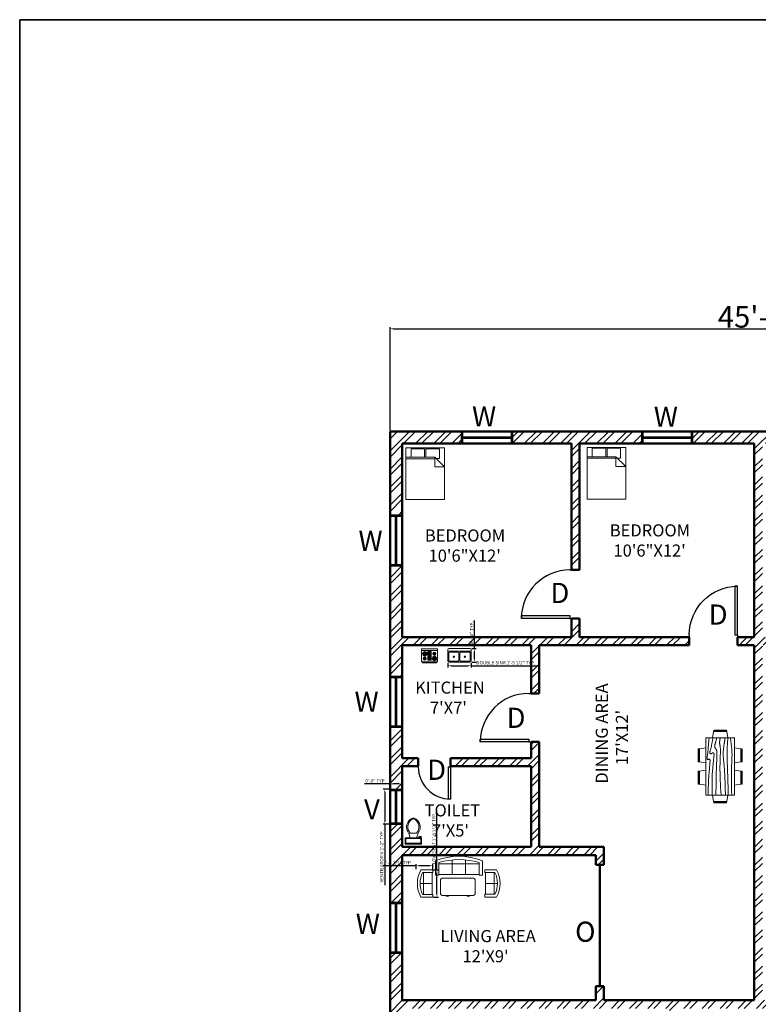
# Model space of a CAD drawing. Units: inches. Extents: x -31485 to -28799, y 18003 to 19130.
# Tile 4 of 15: x -31485 to -30936, y 18398 to 19130. Entities that reach past the tile are written whole.
import ezdxf

# ---------------------------------------------------------------- set-up
doc = ezdxf.new("R2010")
doc.units = ezdxf.units.IN
for name, color, linetype, lineweight in [('A-ANNO-DIMS', 2, 'Continuous', 18), ('A-ANNO-TEXT', 7, 'Continuous', 18), ('A-ANNO-TTLB', 7, 'Continuous', 35), ('A-AREA-IDEN', 7, 'Continuous', 18), ('A-DOOR', 3, 'Continuous', 25), ('A-FLOR-FIXT', 9, 'Continuous', 18), ('A-FURN', 8, 'Continuous', 18), ('A-GLAZ', 4, 'Continuous', 25), ('A-WALL', 7, 'Continuous', 50), ('A-WALL-PATT', 8, 'Continuous', 13)]:
    doc.layers.add(name, color=color, linetype=linetype, lineweight=lineweight)
doc.styles.get("Standard").update_dxf_attribs({"font": 'arial.ttf'})
doc.dimstyles.new('ISO-25', dxfattribs={"dimtxt": 2.5, "dimasz": 2.5, "dimexe": 1.25, "dimexo": 0.625, "dimtad": 1, "dimdec": 0, "dimlunit": 3, "dimtxsty": 'Standard', "dimcen": 2.5, "dimadec": 0, "dimazin": 0, "dimtfac": 1, "dimtdec": 0, "dimtmove": 0, "dimatfit": 3, "dimfxl": 1, "dimarcsym": 0})

# ---------------------------------------------------------------- blocks, each defined once
blk = doc.blocks.new('*U8')
for p, q in [((0, 0), (0, -100)), ((750, 0), (750, -100))]:
    blk.add_line(p, q)
blk.add_lwpolyline([(0, 0), (0, 750), (43.75, 750), (43.75, 0)], close=True)
blk.add_arc((0, 0), 750, 0, 90)
blk = doc.blocks.new('Bed - Queen')
for p, q in [((0, -80.00003), (0, 0)), ((0, 0), (59.99999, 0)), ((59.99999, 0), (59.99999, -80.00003)), ((0, -14.4), (44.8, -14.4)), ((7.99999, -1.2), (28.79998, -1.2)), ((7.99999, -14.4), (7.99999, -1.2)), ((28.79998, -1.2), (28.79998, -14.4)), ((31.19999, -1.2), (51.99999, -1.2)), ((31.19999, -14.4), (31.19999, -1.2)), ((59.99999, -29.6), (44.8, -14.4)), ((44.8, -14.4), (44.8, -29.6)), ((51.99999, -1.2), (51.99999, -16.4)), ((44.8, -16.8), (0, -16.8)), ((44.8, -29.6), (59.99999, -29.6)), ((51.99999, -16.4), (46.79936, -16.4)), ((59.99999, -80.00003), (0, -80.00003))]:
    blk.add_line(p, q)
blk = doc.blocks.new('Desk - 30 x 60 in.')
for p, q in [((-26.999995, 0), (26.999995, 0)), ((-29.999995, -27), (-29.999995, -3)), ((29.999995, -3), (29.999995, -27)), ((26.999995, -30), (-26.999995, -30)), ((-20.000005, -30), (-20.000005, -31)), ((-20.000005, -31), (-16.000005, -31)), ((-16.000005, -31), (-16.000005, -30)), ((15.999995, -31), (15.999995, -30)), ((19.999995, -31), (15.999995, -31)), ((19.999995, -30), (19.999995, -31))]:
    blk.add_line(p, q)
for centre, start, end in [((-26.499995, -3.5), 98.1301, 171.8699), ((26.499995, -3.5), 8.130102, 81.8699), ((-26.499995, -26.5), 188.1301, 261.8699), ((26.499995, -26.5), 278.1301, 351.8699)]:
    blk.add_arc(centre, 3.535534, start, end)
blk = doc.blocks.new('Sofa - Roundback 7 ft.')
for p, q in [((-36.000027, -34), (-36.000027, -11.4696)), ((-35.999844, -13.3819), (35.9998, -13.3819)), ((-12.00002, -32.4421), (-12.00003, -6.5971)), ((11.99997, -32.4421), (11.99998, -6.5971)), ((35.99998, -34), (35.99998, -11.4696)), ((-36.000027, -32.4421), (35.99998, -32.4421))]:
    blk.add_line(p, q)
for points in [[(-36.000027, -34), (-42.000027, -34), (-42.000027, -8)], [(41.99998, -8), (41.99998, -34), (35.99998, -34)]]:
    blk.add_lwpolyline(points)
for centre, radius, start, end in [((0, -114.25), 114.25, 68.43141, 111.5686), ((-0.00001, -127.1968), 121.1968, 72.72033, 107.2797)]:
    blk.add_arc(centre, radius, start, end)
blk = doc.blocks.new('Sofa - Roundback Loveseat 5 ft.')
for p, q in [((-24, -33.99998), (-24, -11.46958)), ((-23.9998, -13.38178), (23.99986, -13.38178)), ((0, -32.44198), (0, -5.99998)), ((24.00004, -33.99998), (24.00004, -11.46958)), ((-24, -32.44198), (24.00004, -32.44198))]:
    blk.add_line(p, q)
for points in [[(-24, -33.99998), (-30, -33.99998), (-30, -7.99998)], [(30.00004, -7.99998), (30.00004, -33.99998), (24.00004, -33.99998)]]:
    blk.add_lwpolyline(points)
for centre, radius, start, end in [((0, -60.24998), 60.24998, 60.13715, 119.8628), ((0, -61.38438), 55.38444, 64.32083, 115.6792)]:
    blk.add_arc(centre, radius, start, end)
blk = doc.blocks.new('Dining Set - 36 x 72 in.')
for p, q in [((-22.2343, 26.00059), (-23.4847, 17.99762)), ((-22.2304, 26), (-5.7608, 26)), ((-22, 27.5), (-22.1562, 26.50042)), ((-5.8416, 26.5), (-22.1534, 26.5)), ((-22, 27.5), (-6, 27.5)), ((-5.8437, 26.49966), (-6, 27.5)), ((-4.5152, 17.99762), (-5.7655, 25.99926)), ((5.7657, 26.00059), (4.5153, 17.99762)), ((5.7696, 26), (22.2392, 26)), ((6, 27.5), (5.8438, 26.50042)), ((22.1584, 26.5), (5.8466, 26.5)), ((6, 27.5), (22, 27.5)), ((22.1563, 26.49966), (22, 27.5)), ((23.4848, 17.99762), (22.2345, 25.99926)), ((36, 18), (-36, 18)), ((-36, 18), (-36, -18)), ((36, -18), (36, 18)), ((-45.5, 8), (-44.5004, 8.15617)), ((-45.5, 8), (-45.5, -8)), ((-44.5, -8.15843), (-44.5, 8.15338)), ((-44.0006, 8.23428), (-35.9976, 9.48474)), ((-44, 8.23041), (-44, -8.23915)), ((44.0006, 8.23428), (35.9976, 9.48474)), ((44, 8.23041), (44, -8.23915)), ((44.5, -8.15843), (44.5, 8.15338)), ((45.5, 8), (44.5005, 8.15617)), ((45.5, 8), (45.5, -8)), ((-44.4997, -8.15631), (-45.5, -8)), ((-35.9976, -9.48476), (-43.9993, -8.2345)), ((35.9976, -9.48476), (43.9993, -8.2345)), ((44.4997, -8.15631), (45.5, -8)), ((-36, -18), (36, -18)), ((-22.2343, -26.0006), (-23.4847, -17.99762)), ((-4.5152, -17.99762), (-5.7655, -25.99928)), ((5.7657, -26.0006), (4.5153, -17.99762)), ((23.4848, -17.99762), (22.2345, -25.99928)), ((-22.2304, -26), (-5.7608, -26)), ((-22, -27.5), (-22.1562, -26.50044)), ((-5.8416, -26.5), (-22.1534, -26.5)), ((-22, -27.5), (-6, -27.5)), ((-5.8437, -26.49967), (-6, -27.5)), ((5.7696, -26), (22.2392, -26)), ((6, -27.5), (5.8438, -26.50044)), ((22.1584, -26.5), (5.8466, -26.5)), ((6, -27.5), (22, -27.5)), ((22.1563, -26.49967), (22, -27.5))]:
    blk.add_line(p, q)
for points in [[(-36, 15), (-31.1772, 14.97754), (-26.8079, 14.91406), (-22.8538, 14.81543), (-19.276, 14.6875), (-16.0362, 14.53613), (-13.0957, 14.36718), (-10.4159, 14.18652), (-7.9583, 14), (-5.6904, 13.81315), (-3.6035, 13.63021), (-1.6954, 13.45508), (0.0365, 13.29166), (1.5945, 13.14388), (2.9811, 13.01562), (4.1988, 12.9108), (5.25, 12.83333), (6.1393, 12.78613), (6.8802, 12.76823), (7.4883, 12.77767), (7.9792, 12.8125), (8.3685, 12.87077), (8.6719, 12.95052), (8.9049, 13.0498), (9.0833, 13.16666), (9.2205, 13.29899), (9.3216, 13.44401), (9.3895, 13.59879), (9.4271, 13.76041), (9.4373, 13.92594), (9.4232, 14.09245), (9.3875, 14.257), (9.3333, 14.41666), (9.2638, 14.56917), (9.1836, 14.71484), (9.0975, 14.85465), (9.0104, 14.98958), (8.9272, 15.1206), (8.8529, 15.2487), (8.7922, 15.37483), (8.75, 15.5), (8.7305, 15.62467), (8.7344, 15.74739), (8.7617, 15.86621), (8.8125, 15.97916), (8.8867, 16.08431), (8.9844, 16.17968), (9.1055, 16.26334), (9.25, 16.33333), (9.4189, 16.38802), (9.6172, 16.42708), (9.8506, 16.45052), (10.125, 16.45833), (10.4463, 16.45052), (10.8203, 16.42708), (11.2529, 16.38802), (11.75, 16.33333), (12.3184, 16.26318), (12.9694, 16.17838), (13.7151, 16.07991), (14.5677, 15.96875), (15.5395, 15.84586), (16.6426, 15.71224), (17.8893, 15.56884), (19.2917, 15.41666), (20.859, 15.25667), (22.5879, 15.08984), (24.4721, 14.91715), (26.5052, 14.73958), (28.6809, 14.5581), (30.9929, 14.3737), (33.4347, 14.18733), (36, 14)], [(-36, 10), (-28.9766, 10.14274), (-23.1725, 10.20442), (-18.4241, 10.19775), (-14.5677, 10.13541), (-11.4399, 10.03011), (-8.877, 9.89453), (-6.7154, 9.74137), (-4.7917, 9.58333), (-2.9698, 9.43082), (-1.2246, 9.28515), (0.4415, 9.14534), (2.026, 9.01041), (3.5266, 8.87939), (4.9408, 8.7513), (6.266, 8.62516), (7.5, 8.5), (8.6411, 8.37549), (9.6914, 8.2539), (10.6538, 8.13818), (11.5312, 8.03125), (12.3267, 7.93603), (13.043, 7.85547), (13.6831, 7.79248), (14.25, 7.75), (14.7471, 7.7303), (15.1797, 7.73307), (15.5537, 7.75732), (15.875, 7.80208), (16.1494, 7.86637), (16.3828, 7.94922), (16.5811, 8.04964), (16.75, 8.16666), (16.8944, 8.29915), (17.0143, 8.44531), (17.1089, 8.60319), (17.1771, 8.77083), (17.218, 8.94629), (17.2305, 9.1276), (17.2137, 9.31282), (17.1667, 9.5), (17.0895, 9.6875), (16.987, 9.875), (16.8649, 10.0625), (16.7292, 10.25), (16.5856, 10.4375), (16.4401, 10.625), (16.2985, 10.8125), (16.1667, 11), (16.05, 11.18733), (15.9518, 11.3737), (15.8752, 11.5581), (15.8229, 11.73958), (15.798, 11.91715), (15.8034, 12.08984), (15.842, 12.25667), (15.9167, 12.41666), (16.0295, 12.56836), (16.1784, 12.70833), (16.3605, 12.83268), (16.5729, 12.9375), (16.8127, 13.01888), (17.0768, 13.07291), (17.3625, 13.0957), (17.6667, 13.08333), (17.9894, 13.03312), (18.3418, 12.94726), (18.7382, 12.82918), (19.1927, 12.68229), (19.7195, 12.51001), (20.3327, 12.31575), (21.0465, 12.10294), (21.875, 11.875), (22.8357, 11.63354), (23.959, 11.37304), (25.2786, 11.08618), (26.8282, 10.76562), (28.6414, 10.40405), (30.752, 9.99414), (33.1936, 9.52856), (36, 9)], [(-36, 5.5), (-30.7157, 5.3348), (-26.069, 5.20963), (-21.9946, 5.11767), (-18.4271, 5.05208), (-15.3009, 5.00602), (-12.5508, 4.97265), (-10.1112, 4.94515), (-7.9167, 4.91666), (-5.909, 4.88167), (-4.0586, 4.83984), (-2.3429, 4.79215), (-0.7396, 4.73958), (0.7739, 4.6831), (2.22, 4.6237), (3.6213, 4.56233), (5, 4.5), (6.373, 4.43782), (7.7344, 4.3776), (9.0723, 4.32129), (10.375, 4.27083), (11.6309, 4.22819), (12.8281, 4.19531), (13.9551, 4.17415), (15, 4.16666), (15.954, 4.17448), (16.819, 4.19791), (17.6001, 4.23698), (18.3021, 4.29166), (18.9299, 4.36198), (19.4883, 4.44791), (19.9823, 4.54948), (20.4167, 4.66666), (20.7969, 4.79899), (21.1302, 4.94401), (21.4245, 5.09879), (21.6875, 5.26041), (21.9271, 5.42594), (22.1511, 5.59245), (22.3672, 5.757), (22.5834, 5.91666), (22.8065, 6.06868), (23.0404, 6.21093), (23.2879, 6.34147), (23.5521, 6.45833), (23.8358, 6.55957), (24.142, 6.64323), (24.4735, 6.70735), (24.8334, 6.75), (25.2235, 6.76969), (25.642, 6.76692), (26.0858, 6.74267), (26.5521, 6.69791), (27.0379, 6.63362), (27.5404, 6.55078), (28.0565, 6.45036), (28.5834, 6.33333), (29.1242, 6.19987), (29.7071, 6.04687), (30.3661, 5.87044), (31.1354, 5.66666), (32.0493, 5.43164), (33.142, 5.16146), (34.4475, 4.85221), (36, 4.5)], [(-36, -1), (-30.7915, -0.6591), (-26.0195, -0.38216), (-21.6519, -0.16284), (-17.6563, 0.00521), (-14.0005, 0.12833), (-10.6523, 0.21289), (-7.5796, 0.26522), (-4.75, 0.29166), (-2.134, 0.29793), (0.2878, 0.28711), (2.5317, 0.26163), (4.6146, 0.22396), (6.5529, 0.17651), (8.3633, 0.12174), (10.0623, 0.06209), (11.6667, 0), (13.1899, -0.06201), (14.6341, -0.1211), (15.9982, -0.17432), (17.2813, -0.21875), (18.4823, -0.25147), (19.6003, -0.26953), (20.6343, -0.27002), (21.5834, -0.25), (22.4481, -0.20768), (23.2357, -0.14584), (23.9549, -0.06836), (24.6146, 0.02083), (25.2235, 0.11784), (25.7904, 0.21875), (26.3241, 0.31966), (26.8334, 0.41666), (27.3265, 0.50618), (27.8099, 0.58593), (28.2894, 0.65397), (28.7709, 0.70833), (29.2601, 0.74707), (29.763, 0.76823), (30.2855, 0.76985), (30.8334, 0.75), (31.4088, 0.70784), (31.9994, 0.64713), (32.589, 0.57275), (33.1615, 0.48958), (33.7008, 0.4025), (34.1908, 0.3164), (34.6153, 0.23616), (34.9584, 0.16666), (35.2099, 0.11165), (35.3848, 0.07031), (35.504, 0.04069), (35.5886, 0.02083), (35.6594, 0.00879), (35.7377, 0.0026), (35.8442, 0.00032), (36, 0)], [(-36, -6.5), (-27.1843, -6.31267), (-20.084, -6.1263), (-14.469, -5.9419), (-10.1094, -5.76042), (-6.7752, -5.58285), (-4.2363, -5.41016), (-2.2629, -5.24333), (-0.625, -5.08334), (0.8708, -4.93099), (2.2715, -4.78646), (3.5872, -4.64974), (4.8281, -4.52084), (6.0046, -4.39974), (7.127, -4.28646), (8.2053, -4.18099), (9.25, -4.08334), (10.2705, -3.99382), (11.2734, -3.91407), (12.2647, -3.84603), (13.25, -3.79167), (14.2354, -3.75293), (15.2266, -3.73177), (16.2295, -3.73015), (17.25, -3.75), (18.2912, -3.79248), (19.3451, -3.85547), (20.4009, -3.93604), (21.4479, -4.03125), (22.4754, -4.13819), (23.4727, -4.25391), (24.4289, -4.37549), (25.3334, -4.5), (26.1785, -4.62492), (26.9694, -4.74935), (27.7145, -4.87281), (28.4219, -4.99479), (29.1, -5.11483), (29.7572, -5.23242), (30.4016, -5.34709), (31.0417, -5.45834), (31.6837, -5.56437), (32.3262, -5.65821), (32.9658, -5.73153), (33.599, -5.77604), (34.2224, -5.78345), (34.8327, -5.74545), (35.4264, -5.65373), (36, -5.5)], [(-36, -10), (-26.4022, -9.81299), (-18.4675, -9.62891), (-11.9839, -9.45069), (-6.7396, -9.28125), (-2.5226, -9.12354), (0.8789, -8.98047), (3.6769, -8.85498), (6.0833, -8.75), (8.2767, -8.66765), (10.3021, -8.60677), (12.1712, -8.56543), (13.8958, -8.54167), (15.4876, -8.53353), (16.9583, -8.53907), (18.3197, -8.55632), (19.5834, -8.58334), (20.7616, -8.61841), (21.8685, -8.66081), (22.9188, -8.71004), (23.9271, -8.76563), (24.9081, -8.82707), (25.8763, -8.89388), (26.8465, -8.96558), (27.8334, -9.04167), (28.8474, -9.12118), (29.8828, -9.20117), (30.93, -9.27824), (31.9792, -9.34896), (33.0205, -9.40991), (34.0443, -9.45768), (35.0407, -9.48885), (36, -9.5)], [(-36, -14.5), (-30.0881, -14.33513), (-25.0332, -14.21224), (-20.7312, -14.12647), (-17.0781, -14.07292), (-13.97, -14.04671), (-11.3027, -14.04297), (-8.9724, -14.05681), (-6.875, -14.08334), (-4.9224, -14.11833), (-3.0905, -14.16016), (-1.3709, -14.20785), (0.2448, -14.26042), (1.7647, -14.3169), (3.1973, -14.3763), (4.5507, -14.43767), (5.8333, -14.5), (7.0554, -14.5621), (8.235, -14.62175), (9.3922, -14.67652), (10.5469, -14.72396), (11.7192, -14.76164), (12.929, -14.78711), (14.1965, -14.79794), (15.5417, -14.79167), (16.9933, -14.76424), (18.6152, -14.70508), (20.4804, -14.60197), (22.6615, -14.44271), (25.2312, -14.21509), (28.2624, -13.9069), (31.8277, -13.50594), (36, -13)]]:
    blk.add_lwpolyline(points)
blk = doc.blocks.new('Range-Oven - 30 in top')
for p, q in [((0, -3), (30, -3)), ((12, -6), (18, -6)), ((13, -20), (13, -6)), ((14, -6), (14, -20)), ((15, -20), (15, -6)), ((16, -6), (16, -20)), ((17, -20), (17, -6)), ((6, -24), (6, -25)), ((8, -25), (8, -24)), ((18, -20), (12, -20)), ((22, -25), (22, -24)), ((24, -24), (24, -25))]:
    blk.add_line(p, q)
for points in [[(0, -24), (0, 0), (30, 0), (30, -24)], [(12, -21), (12, -5), (18, -5), (18, -21)], [(2, -26), (2, -25), (28, -25), (28, -26)]]:
    blk.add_lwpolyline(points, close=True)
for centre, radius in [((6, -9), 4), ((6, -9), 3), ((6, -18), 3), ((6, -9), 2), ((6, -18), 2), ((6, -9), 1), ((6, -18), 1), ((24, -18), 4), ((24, -9), 3), ((24, -18), 3), ((24, -9), 2), ((24, -18), 2), ((24, -9), 1), ((24, -18), 1)]:
    blk.add_circle(centre, radius)
blk = doc.blocks.new('Sink-double - 36 in top')
for p, q in [((-18, -4), (18, -4)), ((-0.75, -18.5), (-0.75, -6.5)), ((0.75, -6.5), (0.75, -18.5))]:
    blk.add_line(p, q)
for points in [[(-16.5, 0), (16.5, 0)], [(-18, -19.5), (-18, -1.5)], [(-16.5, -18.5), (-16.5, -6.5)], [(-15.5, -5.5), (-1.75, -5.5)], [(1.75, -5.5), (15.5, -5.5)], [(16.5, -6.5), (16.5, -18.5)], [(18, -1.5), (18, -19.5)], [(16.5, -21), (-16.5, -21)], [(-1.75, -19.5), (-15.5, -19.5)], [(15.5, -19.5), (1.75, -19.5)]]:
    blk.add_lwpolyline(points)
for centre, radius in [((-8.5, -12.5), 1), ((-8.5, -12.5), 0.5), ((8.5, -12.5), 1), ((8.5, -12.5), 0.5)]:
    blk.add_circle(centre, radius)
for centre, radius, start, end in [((-16.5, -1.5), 1.5, 90, 180), ((16.5, -1.5), 1.5, 0, 90), ((-15.5, -6.5), 1, 90, 180), ((-1.75, -6.5), 1, 0, 90), ((1.75, -6.5), 1, 90, 180), ((15.5, -6.5), 1, 0, 90), ((-16.5, -19.5), 1.5, 180, 270), ((-15.5, -18.5), 1, 180, 270), ((-1.75, -18.5), 1, 270, 0), ((1.75, -18.5), 1, 180, 270), ((15.5, -18.5), 1, 270, 0), ((16.5, -19.5), 1.5, 270, 0)]:
    blk.add_arc(centre, radius, start, end)
blk = doc.blocks.new('Toilet - top')
for p, q in [((-10, -8.5), (-8, -8.5)), ((-10, -9.5), (-10, -8.5)), ((-7, -9.5), (-10, -9.5)), ((-8, -8.5), (-8, -8)), ((-7, -8), (-7, -9.5)), ((-4, -8), (-6, -14)), ((4, -8), (6, -14)), ((9.5, -6), (9.5, -2)), ((4, -14), (-4, -14))]:
    blk.add_line(p, q)
blk.add_lwpolyline([(10.5, -8), (10.5, 0), (-10.5, 0), (-10.5, -8)], close=True)
for points in [[(-9.5, -2), (-9.5, -6)], [(8.5, -1), (-8.5, -1)], [(-8.5, -7), (8.5, -7)]]:
    blk.add_lwpolyline(points)
for centre, radius, start, end in [((-8.6, -1.9), 0.884, 81.8699, 188.1301), ((-8.6, -6.1), 0.884, 171.8699, 278.1301), ((8.6, -1.9), 0.884, 351.8699, 98.1301), ((8.6, -6.1), 0.884, 261.8699, 8.1301), ((3.5, -21.6), 12.2, 141.4691, 247.9714), ((4.2, -21.8), 11.3, 136.3677, 238.9468), ((-3.5, -21.6), 12.2, 292.0284, 38.5307), ((-4.2, -21.8), 11.3, 301.053, 43.6321), ((0, -27.9), 4, 245.7318, 294.2682), ((0, -29), 4, 254.8605, 285.1395)]:
    blk.add_arc(centre, radius, start, end)
blk = doc.blocks.new('*D200')
at = {"layer": 'A-ANNO-DIMS', "color": 0, "lineweight": -2, "transparency": 16777216}
for p, q in [((-31209.53, 18824.43), (-31209.53, 18901.41)), ((-31207.03, 18900.16), (-30664.03, 18900.16)), ((-30661.53, 18824.43), (-30661.53, 18901.41))]:
    blk.add_line(p, q, dxfattribs=at)
at = {"layer": 'A-ANNO-DIMS', "color": 0, "transparency": 16777216}
for points in [[(-31207.03, 18900.58), (-31207.03, 18899.75), (-31209.53, 18900.16)], [(-30664.03, 18900.58), (-30664.03, 18899.75), (-30661.53, 18900.16)]]:
    blk.add_solid(points, dxfattribs=at)
at = {"layer": 'Defpoints', "color": 0, "transparency": 16777216}
for p in [(-30661.53, 18900.16), (-31209.53, 18823.8), (-30661.53, 18823.8)]:
    blk.add_point(p, dxfattribs=at)
at = {"layer": 'A-ANNO-DIMS', "color": 0, "transparency": 16777216, "insert": (-30935.53, 18908.96), "char_height": 2.5, "attachment_point": 5}
blk.add_mtext('{\\H6.4x;45\'-8"}', dxfattribs=at)
blk = doc.blocks.new('WIN-900-W9')
for p, q in [((-29982.21, 18824.12), (-29982.21, 18815.12)), ((-29981.21, 18824.12), (-29981.21, 18815.12)), ((-29945.21, 18824.12), (-29945.21, 18815.12)), ((-29944.21, 18824.12), (-29944.21, 18815.12)), ((-29981.21, 18820.12), (-29945.21, 18820.12)), ((-29981.21, 18819.62), (-29945.21, 18819.62)), ((-29981.21, 18819.12), (-29945.21, 18819.12))]:
    blk.add_line(p, q)
blk = doc.blocks.new('VENT-600-W9')
for p, q in [((-29896.21, 18594.12), (-29905.21, 18594.12)), ((-29896.21, 18593.12), (-29905.21, 18593.12)), ((-29901.21, 18593.12), (-29901.21, 18569.12)), ((-29900.71, 18593.12), (-29900.71, 18569.12)), ((-29900.21, 18593.12), (-29900.21, 18569.12)), ((-29896.21, 18569.12), (-29905.21, 18569.12)), ((-29896.21, 18568.12), (-29905.21, 18568.12))]:
    blk.add_line(p, q)
blk = doc.blocks.new('*D216')
at = {"layer": 'A-ANNO-DIMS', "color": 0, "lineweight": -2, "transparency": 16777216}
for p, q in [((-31210.15, 18557.8), (-31214.68, 18557.8)), ((-31213.43, 18555.3), (-31213.43, 18534.3)), ((-31210.15, 18531.8), (-31214.68, 18531.8)), ((-31213.43, 18531.8), (-31213.43, 18486.49))]:
    blk.add_line(p, q, dxfattribs=at)
at = {"layer": 'A-ANNO-DIMS', "color": 0, "transparency": 16777216}
for points in [[(-31213.84, 18555.3), (-31213.01, 18555.3), (-31213.43, 18557.8)], [(-31213.84, 18534.3), (-31213.01, 18534.3), (-31213.43, 18531.8)]]:
    blk.add_solid(points, dxfattribs=at)
at = {"layer": 'Defpoints', "color": 0, "transparency": 16777216}
for p in [(-31209.53, 18557.8), (-31213.43, 18531.8), (-31209.53, 18531.8)]:
    blk.add_point(p, dxfattribs=at)
at = {"layer": 'A-ANNO-DIMS', "color": 0, "transparency": 16777216, "insert": (-31215.35, 18507.89), "char_height": 2.5, "attachment_point": 5, "rotation": 90}
blk.add_mtext('VENTILATOR V 2\'-2" TYP.', dxfattribs=at)
blk = doc.blocks.new('*D217')
at = {"layer": 'A-ANNO-DIMS', "color": 0, "lineweight": -2, "transparency": 16777216}
for p, q in [((-31209.53, 18561.7), (-31228.52, 18561.7)), ((-31209.53, 18558.43), (-31209.53, 18562.95)), ((-31203.03, 18561.7), (-31207.03, 18561.7)), ((-31200.53, 18558.43), (-31200.53, 18562.95))]:
    blk.add_line(p, q, dxfattribs=at)
at = {"layer": 'A-ANNO-DIMS', "color": 0, "transparency": 16777216}
for points in [[(-31207.03, 18562.12), (-31207.03, 18561.29), (-31209.53, 18561.7)], [(-31203.03, 18562.12), (-31203.03, 18561.29), (-31200.53, 18561.7)]]:
    blk.add_solid(points, dxfattribs=at)
at = {"layer": 'Defpoints', "color": 0, "transparency": 16777216}
for p in [(-31209.53, 18561.7), (-31209.53, 18557.8), (-31200.53, 18557.8)]:
    blk.add_point(p, dxfattribs=at)
at = {"layer": 'A-ANNO-DIMS', "color": 0, "transparency": 16777216, "insert": (-31220.27, 18563.6), "char_height": 2.5, "attachment_point": 5}
blk.add_mtext('0\'-9" TYP.', dxfattribs=at)
blk = doc.blocks.new('*D226')
at = {"layer": 'A-ANNO-DIMS', "color": 0, "lineweight": -2, "transparency": 16777216}
for p, q in [((-31174.67, 18497.78), (-31174.67, 18541.89)), ((-31177.09, 18497.78), (-31173.42, 18497.78)), ((-31174.67, 18479.99), (-31174.67, 18495.28)), ((-31177.09, 18477.49), (-31173.42, 18477.49))]:
    blk.add_line(p, q, dxfattribs=at)
at = {"layer": 'A-ANNO-DIMS', "color": 0, "transparency": 16777216}
for points in [[(-31175.08, 18495.28), (-31174.25, 18495.28), (-31174.67, 18497.78)], [(-31175.08, 18479.99), (-31174.25, 18479.99), (-31174.67, 18477.49)]]:
    blk.add_solid(points, dxfattribs=at)
at = {"layer": 'Defpoints', "color": 0, "transparency": 16777216}
for p in [(-31177.71, 18497.78), (-31174.67, 18497.78), (-31177.71, 18477.49)]:
    blk.add_point(p, dxfattribs=at)
at = {"layer": 'A-ANNO-DIMS', "color": 0, "transparency": 16777216, "insert": (-31176.59, 18521.08), "char_height": 2.5, "attachment_point": 5, "rotation": 90}
blk.add_mtext('LOVESEAT 1\'-8 1/2" TYP.', dxfattribs=at)
blk = doc.blocks.new('*D227')
at = {"layer": 'A-ANNO-DIMS', "color": 0, "lineweight": -2, "transparency": 16777216}
for p, q in [((-31190.11, 18498.4), (-31190.11, 18502.07)), ((-31177.71, 18498.4), (-31177.71, 18502.07)), ((-31190.11, 18500.82), (-31214.69, 18500.82)), ((-31180.21, 18500.82), (-31187.61, 18500.82))]:
    blk.add_line(p, q, dxfattribs=at)
at = {"layer": 'A-ANNO-DIMS', "color": 0, "transparency": 16777216}
for points in [[(-31187.61, 18501.24), (-31187.61, 18500.4), (-31190.11, 18500.82)], [(-31180.21, 18501.24), (-31180.21, 18500.4), (-31177.71, 18500.82)]]:
    blk.add_solid(points, dxfattribs=at)
at = {"layer": 'Defpoints', "color": 0, "transparency": 16777216}
for p in [(-31190.11, 18500.82), (-31190.11, 18497.78), (-31177.71, 18497.78)]:
    blk.add_point(p, dxfattribs=at)
at = {"layer": 'A-ANNO-DIMS', "color": 0, "transparency": 16777216, "insert": (-31203.65, 18502.74), "char_height": 2.5, "attachment_point": 5}
blk.add_mtext('1\'-0 1/2" TYP.', dxfattribs=at)
blk = doc.blocks.new('*D254')
at = {"layer": 'A-ANNO-DIMS', "color": 0, "lineweight": -2, "transparency": 16777216}
for p, q in [((-31166.61, 18651.53), (-31166.61, 18648.3)), ((-31164.11, 18649.55), (-31151.75, 18649.55)), ((-31149.25, 18651.53), (-31149.25, 18648.3)), ((-31149.25, 18649.55), (-31100.1, 18649.55))]:
    blk.add_line(p, q, dxfattribs=at)
at = {"layer": 'A-ANNO-DIMS', "color": 0, "transparency": 16777216}
for points in [[(-31164.11, 18649.96), (-31164.11, 18649.13), (-31166.61, 18649.55)], [(-31151.75, 18649.96), (-31151.75, 18649.13), (-31149.25, 18649.55)]]:
    blk.add_solid(points, dxfattribs=at)
at = {"layer": 'Defpoints', "color": 0, "transparency": 16777216}
for p in [(-31166.61, 18652.15), (-31149.25, 18652.15), (-31149.25, 18649.55)]:
    blk.add_point(p, dxfattribs=at)
at = {"layer": 'A-ANNO-DIMS', "color": 0, "transparency": 16777216, "insert": (-31123.42, 18651.46), "char_height": 2.5, "attachment_point": 5}
blk.add_mtext('DOUBLE SINK 1\'-5 1/2" TYP.', dxfattribs=at)
blk = doc.blocks.new('*D255')
at = {"layer": 'A-ANNO-DIMS', "color": 0, "lineweight": -2, "transparency": 16777216}
for p, q in [((-31146.64, 18662.28), (-31146.64, 18683.21)), ((-31148.62, 18662.28), (-31145.39, 18662.28)), ((-31146.64, 18654.65), (-31146.64, 18659.78)), ((-31148.62, 18652.15), (-31145.39, 18652.15))]:
    blk.add_line(p, q, dxfattribs=at)
at = {"layer": 'A-ANNO-DIMS', "color": 0, "transparency": 16777216}
for points in [[(-31147.06, 18659.78), (-31146.23, 18659.78), (-31146.64, 18662.28)], [(-31147.06, 18654.65), (-31146.23, 18654.65), (-31146.64, 18652.15)]]:
    blk.add_solid(points, dxfattribs=at)
at = {"layer": 'Defpoints', "color": 0, "transparency": 16777216}
for p in [(-31149.25, 18662.28), (-31146.64, 18662.28), (-31149.25, 18652.15)]:
    blk.add_point(p, dxfattribs=at)
at = {"layer": 'A-ANNO-DIMS', "color": 0, "transparency": 16777216, "insert": (-31148.54, 18674), "char_height": 2.5, "attachment_point": 5, "rotation": 90}
blk.add_mtext('0\'-10" TYP.', dxfattribs=at)

msp = doc.modelspace()

# ---------------------------------------------------------------- hatches: boundary and pattern name
at = {"layer": 'A-WALL-PATT'}
h = msp.add_hatch(dxfattribs=at)
h.set_pattern_fill('ANSI32', color=256)
h.set_pattern_definition([(45, (-1687.357, -0.313), (-6.735192, 6.735192), []), (45, (-1682.867, -0.313), (-6.735192, 6.735192), [])])
h.paths.add_polyline_path([(-31156.53, 18823.8), (-31209.53, 18823.8), (-31209.53, 18761.8), (-31200.53, 18761.8), (-31200.53, 18814.8), (-31156.53, 18814.8)], flags=17)
h.paths.add_polyline_path([(-31022.53, 18823.8), (-31118.53, 18823.8), (-31118.53, 18814.8), (-31074.53, 18814.8), (-31074.53, 18720.79), (-31070.96, 18720.79), (-31068.53, 18720.76), (-31068.53, 18814.8), (-31022.53, 18814.8)], flags=17)
h.paths.add_polyline_path([(-30754.53, 18823.8), (-30850.53, 18823.8), (-30850.53, 18814.8), (-30806.53, 18814.8), (-30806.53, 18723.1), (-30800.53, 18723.1), (-30800.53, 18814.8), (-30754.53, 18814.8)], flags=17)
h.paths.add_polyline_path([(-30661.53, 18823.8), (-30716.53, 18823.8), (-30716.53, 18814.8), (-30670.53, 18814.8), (-30670.53, 18761.8), (-30661.53, 18761.8)], flags=17)
h.paths.add_polyline_path([(-30986.92, 18670.8), (-31068.53, 18670.8), (-31068.53, 18684.76), (-31074.53, 18684.76), (-31074.53, 18670.8), (-31200.53, 18670.8), (-31200.53, 18723.8), (-31209.53, 18723.8), (-31209.53, 18641.8), (-31200.53, 18641.8), (-31200.53, 18664.8), (-31104.53, 18664.8), (-31104.53, 18628.93), (-31098.53, 18628.93), (-31098.53, 18664.8), (-30986.92, 18664.8)], flags=17)
h.paths.add_polyline_path([(-30661.53, 18723.8), (-30670.53, 18723.8), (-30670.53, 18670.8), (-30800.53, 18670.8), (-30800.53, 18687.1), (-30806.53, 18687.1), (-30806.53, 18670.8), (-30885.6, 18670.8), (-30885.6, 18667.8), (-30885.6, 18664.8), (-30760.53, 18664.8), (-30760.53, 18625.8), (-30754.53, 18625.8), (-30754.53, 18664.8), (-30670.53, 18664.8), (-30670.53, 18641.8), (-30661.53, 18641.8)], flags=17)
h.paths.add_polyline_path([(-31200.53, 18574.8), (-31188.56, 18574.8), (-31188.56, 18580.8), (-31200.53, 18580.8), (-31200.53, 18603.8), (-31209.53, 18603.8), (-31209.53, 18557.8), (-31200.53, 18557.8)], flags=17)
h.paths.add_polyline_path([(-31098.53, 18592.93), (-31104.53, 18592.93), (-31104.53, 18580.8), (-31164.56, 18580.8), (-31164.56, 18574.8), (-31104.53, 18574.8), (-31104.53, 18514.8), (-31200.53, 18514.8), (-31200.53, 18531.8), (-31209.53, 18531.8), (-31209.53, 18473.8), (-31200.53, 18473.8), (-31200.53, 18508.8), (-31056.53, 18508.8), (-31056.53, 18501.62), (-31050.53, 18501.62), (-31050.53, 18514.8), (-31098.53, 18514.8)], flags=17)
h.paths.add_polyline_path([(-30661.53, 18531.8), (-30670.53, 18531.8), (-30670.53, 18514.8), (-30754.53, 18514.8), (-30754.53, 18574.8), (-30700.75, 18574.8), (-30700.75, 18577.44), (-30700.75, 18580.8), (-30754.53, 18580.8), (-30754.53, 18589.8), (-30760.53, 18589.8), (-30760.53, 18514.8), (-30820.53, 18514.8), (-30820.53, 18499.26), (-30814.53, 18499.26), (-30814.53, 18508.8), (-30670.53, 18508.8), (-30670.53, 18473.8), (-30661.53, 18473.8)], flags=17)
h.paths.add_polyline_path([(-30661.53, 18435.8), (-30670.53, 18435.8), (-30670.53, 18400.8), (-30814.53, 18400.8), (-30814.53, 18413.15), (-30820.53, 18413.15), (-30820.53, 18400.8), (-30932.53, 18400.8), (-30932.53, 18664.8), (-30921.6, 18664.8), (-30921.6, 18670.8), (-30932.53, 18670.8), (-30932.53, 18814.8), (-30888.53, 18814.8), (-30888.53, 18823.8), (-30984.53, 18823.8), (-30984.53, 18814.8), (-30938.53, 18814.8), (-30938.53, 18670.8), (-30950.92, 18670.8), (-30950.92, 18664.8), (-30938.53, 18664.8), (-30938.53, 18400.8), (-31050.53, 18400.8), (-31050.53, 18411.18), (-31056.53, 18411.18), (-31056.53, 18400.8), (-31200.53, 18400.8), (-31200.53, 18435.8), (-31209.53, 18435.8), (-31209.53, 18179.8), (-31200.53, 18179.8), (-31200.53, 18394.8), (-31001.53, 18394.8), (-31001.53, 18179.8), (-30954.53, 18179.8), (-30954.53, 18188.8), (-30995.53, 18188.8), (-30995.53, 18394.8), (-30875.53, 18394.8), (-30875.53, 18188.8), (-30916.53, 18188.8), (-30916.53, 18179.8), (-30869.53, 18179.8), (-30869.53, 18394.8), (-30670.53, 18394.8), (-30670.53, 18179.8), (-30661.53, 18179.8)])

# ---------------------------------------------------------------- linework, layer by layer
at = {"layer": 'A-ANNO-TTLB'}
msp.add_lwpolyline([(-31485.1, 19129.94), (-28798.64, 19129.94), (-28798.64, 18002.86), (-31485.1, 18002.86)], close=True, dxfattribs=at)
at = {"layer": 'A-WALL'}
for p, q in [((-31209.53, 18823.8), (-30661.53, 18823.8)), ((-31209.53, 18179.8), (-31209.53, 18823.8)), ((-31200.53, 18814.8), (-31074.53, 18814.8)), ((-31200.53, 18670.8), (-31200.53, 18814.8)), ((-31074.53, 18720.76), (-31074.53, 18814.8)), ((-31068.53, 18814.8), (-30938.53, 18814.8)), ((-31068.53, 18720.76), (-31068.53, 18814.8)), ((-30938.53, 18814.8), (-30938.53, 18670.8)), ((-31074.53, 18720.76), (-31068.53, 18720.76)), ((-31074.53, 18670.8), (-31074.53, 18684.76)), ((-31074.53, 18684.76), (-31068.53, 18684.76)), ((-31068.53, 18670.8), (-31068.53, 18684.76)), ((-31200.53, 18670.8), (-31074.53, 18670.8)), ((-31068.53, 18670.8), (-30986.92, 18670.8)), ((-30986.92, 18670.8), (-30986.92, 18664.8)), ((-30950.92, 18670.8), (-30938.53, 18670.8)), ((-30950.92, 18670.8), (-30950.92, 18664.8)), ((-31200.53, 18664.8), (-31104.53, 18664.8)), ((-31200.53, 18580.8), (-31200.53, 18664.8)), ((-31104.53, 18628.93), (-31104.53, 18664.8)), ((-31098.53, 18664.8), (-30986.92, 18664.8)), ((-31098.53, 18628.93), (-31098.53, 18664.8)), ((-30950.92, 18664.8), (-30938.53, 18664.8)), ((-30938.53, 18664.8), (-30938.53, 18400.8)), ((-31104.53, 18628.93), (-31098.53, 18628.93)), ((-31104.53, 18580.8), (-31104.53, 18592.93)), ((-31104.53, 18592.93), (-31098.53, 18592.93)), ((-31098.53, 18514.8), (-31098.53, 18592.93)), ((-31200.53, 18580.8), (-31188.56, 18580.8)), ((-31200.53, 18574.8), (-31188.56, 18574.8)), ((-31200.53, 18514.8), (-31200.53, 18574.8)), ((-31188.56, 18580.8), (-31188.56, 18574.8)), ((-31164.56, 18580.8), (-31104.53, 18580.8)), ((-31164.56, 18580.8), (-31164.56, 18574.8)), ((-31164.56, 18574.8), (-31104.53, 18574.8)), ((-31104.53, 18514.8), (-31104.53, 18574.8)), ((-31200.53, 18514.8), (-31104.53, 18514.8)), ((-31200.53, 18508.8), (-31056.53, 18508.8)), ((-31200.53, 18400.8), (-31200.53, 18508.8)), ((-31098.53, 18514.8), (-31050.53, 18514.8)), ((-31056.53, 18501.62), (-31056.53, 18508.8)), ((-31050.53, 18501.62), (-31050.53, 18514.8)), ((-31056.53, 18501.62), (-31050.53, 18501.62)), ((-31053.53, 18501.62), (-31053.53, 18411.18)), ((-31056.53, 18400.8), (-31056.53, 18411.18)), ((-31056.53, 18411.18), (-31050.53, 18411.18)), ((-31050.53, 18400.8), (-31050.53, 18411.18)), ((-31200.53, 18400.8), (-31056.53, 18400.8)), ((-31050.53, 18400.8), (-30938.53, 18400.8))]:
    msp.add_line(p, q, dxfattribs=at)

# ---------------------------------------------------------------- block references
at = {"layer": 'A-DOOR'}
for p, xscale, yscale, zscale, rotation in [((-31075.76, 18684.74), 0.0480636078261425, 0.0480636078261425, 0.0480636078261425, 90.00000000000003), ((-31106.36, 18592.92), 0.0480122828236164, 0.0480122828236164, 0.0480122828236164, 90.00000000000003), ((-31164.56, 18574.45), 0.0319880955261889, 0.0319880955261889, 0.0319880955261889, 180)]:
    msp.add_blockref('*U8', p, dxfattribs=dict(at, xscale=xscale, yscale=yscale, zscale=zscale, rotation=rotation))
at = {"layer": 'A-DOOR', "xscale": -0.0480000000000013, "yscale": 0.0480000000000013, "zscale": 0.0480000000000013}
msp.add_blockref('*U8', (-30950.92, 18672.6), dxfattribs=at)
at = {"layer": 'A-FLOR-FIXT'}
for name, p, xscale, yscale, zscale in [('Sink-double - 36 in top', (-31157.93, 18662.28), 0.4823765274114516, 0.4823765274114516, 0.4823765274114516), ('Range-Oven - 30 in top', (-31186.15, 18662.06), 0.4, 0.4, 0.4)]:
    msp.add_blockref(name, p, dxfattribs=dict(at, xscale=xscale, yscale=yscale, zscale=zscale))
at = {"layer": 'A-FLOR-FIXT', "xscale": 0.5850068734066302, "yscale": 0.5850068734066302, "zscale": 0.5850068734066302, "rotation": 180}
msp.add_blockref('Toilet - top', (-31192.16, 18516.94), dxfattribs=at)
at = {"layer": 'A-FURN'}
for name, p, xscale, yscale, zscale in [('Bed - Queen', (-31197.75, 18811.54), 0.479364226334794, 0.479364226334794, 0.479364226334794), ('Bed - Queen', (-31062.9, 18811.85), 0.479364226334794, 0.479364226334794, 0.479364226334794), ('Sofa - Roundback 7 ft.', (-31158.28, 18507.9), 0.4147575827902149, 0.4147575827902149, 0.4147575827902149), ('Desk - 30 x 60 in.', (-31159.11, 18491.59), 0.4297812202416646, 0.4297812202416646, 0.4297812202416646)]:
    msp.add_blockref(name, p, dxfattribs=dict(at, xscale=xscale, yscale=yscale, zscale=zscale))
for name, p, xscale, yscale, zscale, rotation in [('Dining Set - 36 x 72 in.', (-30963.88, 18574.61), 0.5930176886900861, 0.5930176886900861, 0.5930176886900861, 90), ('Sofa - Roundback Loveseat 5 ft.', (-31189.21, 18487.63), 0.3381495698466857, 0.3381495698466857, 0.3381495698466857, 89.99999999999999), ('Sofa - Roundback Loveseat 5 ft.', (-31127.6, 18487.71), 0.3381495698466857, 0.3381495698466857, 0.3381495698466857, 270)]:
    msp.add_blockref(name, p, dxfattribs=dict(at, xscale=xscale, yscale=yscale, zscale=zscale, rotation=rotation))
at = {"layer": 'A-GLAZ'}
for p in [(-1174.32, -0.31), (-1040.32, -0.31)]:
    msp.add_blockref('WIN-900-W9', p, dxfattribs=at)
for name, p, rotation in [('WIN-900-W9', (-12385.41, 48706.01), 89.99999999997677), ('WIN-900-W9', (-12385.41, 48586.01), 89.9999999999743), ('VENT-600-W9', (-61105.73, 37125.92), 180), ('WIN-900-W9', (-12385.41, 48418.01), 89.9999999999743)]:
    msp.add_blockref(name, p, dxfattribs=dict(at, rotation=rotation))

# ---------------------------------------------------------------- texts
at = {"layer": 'A-ANNO-TEXT', "char_height": 15, "attachment_point": 1}
for s, insert in [('{W}', (-31148.54, 18842.45)), ('{W}', (-31013.31, 18842.27)), ('{W}', (-31233.02, 18749.96)), ('{D}', (-31090.22, 18711.18)), ('{D}', (-30972.48, 18695.11)), ('{W}', (-31235.96, 18630.31)), ('{D}', (-31122.85, 18618.32)), ('{D}', (-31181.91, 18579.69)), ('{V}', (-31228.9, 18550.31)), ('{W}', (-31235.05, 18465.2)), ('{O}', (-31071.83, 18459.28))]:
    msp.add_mtext_dynamic_manual_height_columns(s, width=638.549, gutter_width=12.5, heights=[0], dxfattribs=dict(at, insert=insert))
at = {"layer": 'A-AREA-IDEN', "char_height": 9, "attachment_point": 1}
for s, insert in [('{BEDROOM\\P 10\'6"X12\'}', (-31183.61, 18750.91)), ('{BEDROOM\\P 10\'6"X12\'}', (-31046.03, 18754.71)), ("{ KITCHEN\\P     7'X7'}", (-31193.59, 18637.82)), ("{TOILET\\P  7'X5'}", (-31183.79, 18546.53)), ("{LIVING AREA\\P      12'X9'}", (-31172.12, 18453.04))]:
    msp.add_mtext_dynamic_manual_height_columns(s, width=763.1479, gutter_width=12.5, heights=[0], dxfattribs=dict(at, insert=insert))
at = {"layer": 'A-AREA-IDEN', "insert": (-31056.49, 18561.87), "char_height": 9, "attachment_point": 1, "rotation": 90}
msp.add_mtext_dynamic_manual_height_columns("{DINING AREA\\P     17'X12'}", width=763.1479, gutter_width=12.5, heights=[0], dxfattribs=at)

# ---------------------------------------------------------------- dimensions: what is measured, and where the dimension line sits
at = {"layer": 'A-ANNO-DIMS'}
for base, p1, p2, text, override, picture, middle in [((-30661.53, 18900.16), (-31209.53, 18823.8), (-30661.53, 18823.8), '{\\H6.4x;<>}', {"dimclrd": 0, "dimclre": 0, "dimclrt": 0}, '*D200', (-30935.53, 18908.96)), ((-31149.25, 18649.55), (-31166.61, 18652.15), (-31149.25, 18652.15), 'DOUBLE SINK <> TYP.', {"dimdec": 1, "dimlfac": 1, "dimrnd": 0, "dimzin": 1, "dimdsep": 46, "dimlunit": 4, "dimfrac": 2}, '*D254', (-31123.42, 18651.46))]:
    dim = msp.add_linear_dim(base=base, p1=p1, p2=p2, text=text, dimstyle='ISO-25', override=override, dxfattribs=at)
    dim.commit()
    dim.dimension.update_dxf_attribs({"geometry": picture, "text_midpoint": middle})
for base, p1, p2, angle, text, picture, middle in [((-31146.64, 18662.28), (-31149.25, 18652.15), (-31149.25, 18662.28), 90, '<> TYP.', '*D255', (-31148.54, 18674)), ((-31209.53, 18561.7), (-31200.53, 18557.8), (-31209.53, 18557.8), 180, '<> TYP.', '*D217', (-31220.27, 18563.6)), ((-31213.43, 18531.8), (-31209.53, 18557.8), (-31209.53, 18531.8), 270, 'VENTILATOR V <> TYP.', '*D216', (-31215.35, 18507.89)), ((-31174.67, 18497.78), (-31177.71, 18477.49), (-31177.71, 18497.78), 90, 'LOVESEAT <> TYP.', '*D226', (-31176.59, 18521.08)), ((-31190.11, 18500.82), (-31177.71, 18497.78), (-31190.11, 18497.78), 180, '<> TYP.', '*D227', (-31203.65, 18502.74))]:
    dim = msp.add_linear_dim(base=base, p1=p1, p2=p2, angle=angle, text=text, dimstyle='ISO-25', override={"dimdec": 1, "dimlfac": 1, "dimrnd": 0, "dimzin": 1, "dimdsep": 46, "dimlunit": 4, "dimfrac": 2}, dxfattribs=at)
    dim.commit()
    dim.dimension.update_dxf_attribs({"geometry": picture, "text_midpoint": middle})

doc.saveas('drawing.dxf')
